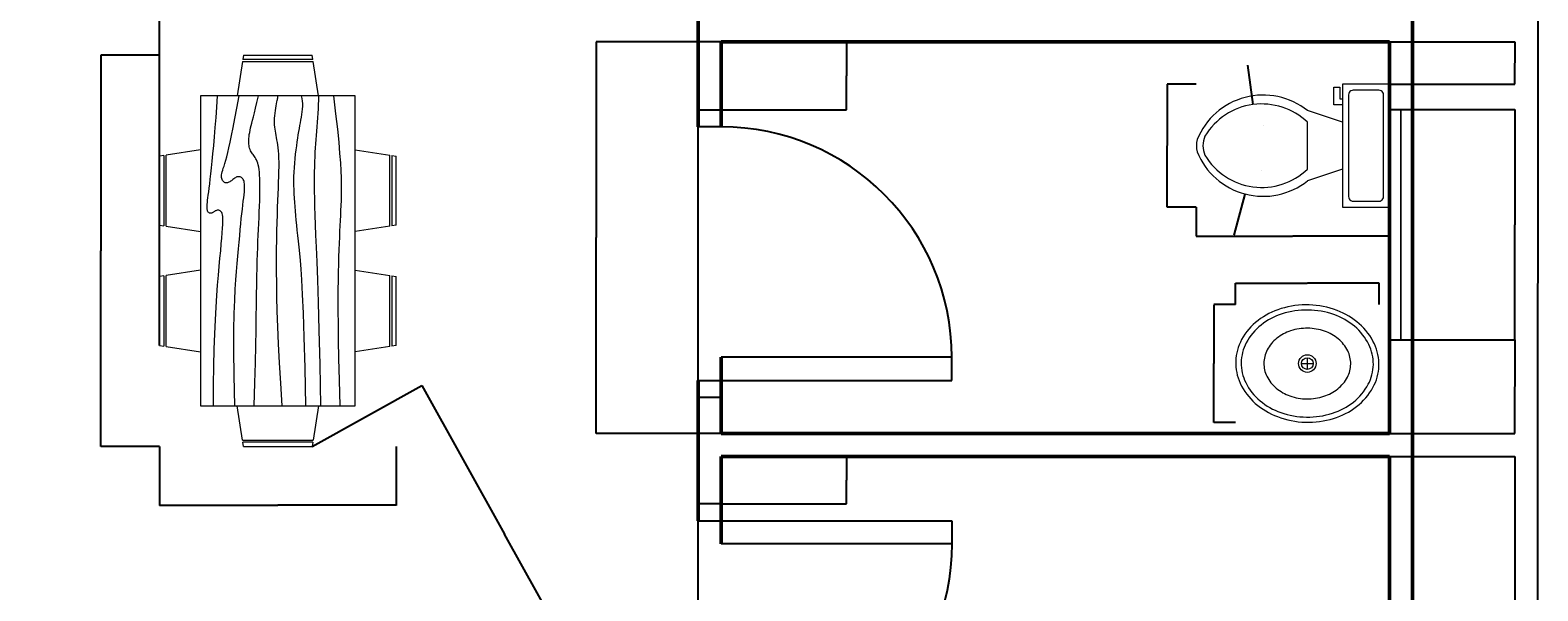
# Model space of a CAD drawing. Units: millimetres. Extents: x 1584 to 12772, y -932 to 10602.
# Tile 3 of 4: x 6228 to 12772, y 3427 to 5860. Entities that reach past the tile are written whole.
import ezdxf

# ---------------------------------------------------------------- set-up
doc = ezdxf.new("R2010")
doc.units = ezdxf.units.MM
for name, color, linetype, lineweight in [('A-ANNO-DIMS', 2, 'Continuous', 18), ('A-DOOR', 3, 'Continuous', 25), ('A-FLOR-FIXT', 9, 'Continuous', 18), ('A-FURN', 8, 'Continuous', 18), ('A-GLAZ', 4, 'Continuous', 18), ('A-WALL', 7, 'Continuous', 50)]:
    doc.layers.add(name, color=color, linetype=linetype, lineweight=lineweight)
doc.styles.get("Standard").update_dxf_attribs({"font": 'arial.ttf'})
doc.dimstyles.get("Standard").update_dxf_attribs({"dimtxt": 0.18, "dimasz": 0.18, "dimexe": 0.18, "dimexo": 0.0625, "dimgap": 0.09, "dimtad": 0, "dimtih": 1, "dimtoh": 1, "dimdec": 4, "dimzin": 0, "dimdsep": 46, "dimtxsty": 'Standard', "dimcen": 0.09, "dimadec": 0, "dimazin": 0, "dimtfac": 1, "dimtdec": 4, "dimtofl": 0, "dimtmove": 0, "dimatfit": 3, "dimfxl": 1, "dimtolj": 1, "dimtzin": 0, "dimarcsym": 0})

# ---------------------------------------------------------------- blocks, each defined once
blk = doc.blocks.new('Dining Set - 36 x 72 in.')
for p, q in [((-22.2343, 26.00059), (-23.4847, 17.99762)), ((-22.2304, 26), (-5.7608, 26)), ((-22, 27.5), (-22.1562, 26.50042)), ((-5.8416, 26.5), (-22.1534, 26.5)), ((-22, 27.5), (-6, 27.5)), ((-5.8437, 26.49966), (-6, 27.5)), ((-4.5152, 17.99762), (-5.7655, 25.99926)), ((5.7657, 26.00059), (4.5153, 17.99762)), ((5.7696, 26), (22.2392, 26)), ((6, 27.5), (5.8438, 26.50042)), ((22.1584, 26.5), (5.8466, 26.5)), ((6, 27.5), (22, 27.5)), ((22.1563, 26.49966), (22, 27.5)), ((23.4848, 17.99762), (22.2345, 25.99926)), ((36, 18), (-36, 18)), ((-36, 18), (-36, -18)), ((36, -18), (36, 18)), ((-45.5, 8), (-44.5004, 8.15617)), ((-45.5, 8), (-45.5, -8)), ((-44.5, -8.15843), (-44.5, 8.15338)), ((-44.0006, 8.23428), (-35.9976, 9.48474)), ((-44, 8.23041), (-44, -8.23915)), ((44.0006, 8.23428), (35.9976, 9.48474)), ((44, 8.23041), (44, -8.23915)), ((44.5, -8.15843), (44.5, 8.15338)), ((45.5, 8), (44.5005, 8.15617)), ((45.5, 8), (45.5, -8)), ((-44.4997, -8.15631), (-45.5, -8)), ((-35.9976, -9.48476), (-43.9993, -8.2345)), ((35.9976, -9.48476), (43.9993, -8.2345)), ((44.4997, -8.15631), (45.5, -8)), ((-36, -18), (36, -18)), ((-22.2343, -26.0006), (-23.4847, -17.99762)), ((-4.5152, -17.99762), (-5.7655, -25.99928)), ((5.7657, -26.0006), (4.5153, -17.99762)), ((23.4848, -17.99762), (22.2345, -25.99928)), ((-22.2304, -26), (-5.7608, -26)), ((-22, -27.5), (-22.1562, -26.50044)), ((-5.8416, -26.5), (-22.1534, -26.5)), ((-22, -27.5), (-6, -27.5)), ((-5.8437, -26.49967), (-6, -27.5)), ((5.7696, -26), (22.2392, -26)), ((6, -27.5), (5.8438, -26.50044)), ((22.1584, -26.5), (5.8466, -26.5)), ((6, -27.5), (22, -27.5)), ((22.1563, -26.49967), (22, -27.5))]:
    blk.add_line(p, q)
for points in [[(-36, 15), (-31.1772, 14.97754), (-26.8079, 14.91406), (-22.8538, 14.81543), (-19.276, 14.6875), (-16.0362, 14.53613), (-13.0957, 14.36718), (-10.4159, 14.18652), (-7.9583, 14), (-5.6904, 13.81315), (-3.6035, 13.63021), (-1.6954, 13.45508), (0.0365, 13.29166), (1.5945, 13.14388), (2.9811, 13.01562), (4.1988, 12.9108), (5.25, 12.83333), (6.1393, 12.78613), (6.8802, 12.76823), (7.4883, 12.77767), (7.9792, 12.8125), (8.3685, 12.87077), (8.6719, 12.95052), (8.9049, 13.0498), (9.0833, 13.16666), (9.2205, 13.29899), (9.3216, 13.44401), (9.3895, 13.59879), (9.4271, 13.76041), (9.4373, 13.92594), (9.4232, 14.09245), (9.3875, 14.257), (9.3333, 14.41666), (9.2638, 14.56917), (9.1836, 14.71484), (9.0975, 14.85465), (9.0104, 14.98958), (8.9272, 15.1206), (8.8529, 15.2487), (8.7922, 15.37483), (8.75, 15.5), (8.7305, 15.62467), (8.7344, 15.74739), (8.7617, 15.86621), (8.8125, 15.97916), (8.8867, 16.08431), (8.9844, 16.17968), (9.1055, 16.26334), (9.25, 16.33333), (9.4189, 16.38802), (9.6172, 16.42708), (9.8506, 16.45052), (10.125, 16.45833), (10.4463, 16.45052), (10.8203, 16.42708), (11.2529, 16.38802), (11.75, 16.33333), (12.3184, 16.26318), (12.9694, 16.17838), (13.7151, 16.07991), (14.5677, 15.96875), (15.5395, 15.84586), (16.6426, 15.71224), (17.8893, 15.56884), (19.2917, 15.41666), (20.859, 15.25667), (22.5879, 15.08984), (24.4721, 14.91715), (26.5052, 14.73958), (28.6809, 14.5581), (30.9929, 14.3737), (33.4347, 14.18733), (36, 14)], [(-36, 10), (-28.9766, 10.14274), (-23.1725, 10.20442), (-18.4241, 10.19775), (-14.5677, 10.13541), (-11.4399, 10.03011), (-8.877, 9.89453), (-6.7154, 9.74137), (-4.7917, 9.58333), (-2.9698, 9.43082), (-1.2246, 9.28515), (0.4415, 9.14534), (2.026, 9.01041), (3.5266, 8.87939), (4.9408, 8.7513), (6.266, 8.62516), (7.5, 8.5), (8.6411, 8.37549), (9.6914, 8.2539), (10.6538, 8.13818), (11.5312, 8.03125), (12.3267, 7.93603), (13.043, 7.85547), (13.6831, 7.79248), (14.25, 7.75), (14.7471, 7.7303), (15.1797, 7.73307), (15.5537, 7.75732), (15.875, 7.80208), (16.1494, 7.86637), (16.3828, 7.94922), (16.5811, 8.04964), (16.75, 8.16666), (16.8944, 8.29915), (17.0143, 8.44531), (17.1089, 8.60319), (17.1771, 8.77083), (17.218, 8.94629), (17.2305, 9.1276), (17.2137, 9.31282), (17.1667, 9.5), (17.0895, 9.6875), (16.987, 9.875), (16.8649, 10.0625), (16.7292, 10.25), (16.5856, 10.4375), (16.4401, 10.625), (16.2985, 10.8125), (16.1667, 11), (16.05, 11.18733), (15.9518, 11.3737), (15.8752, 11.5581), (15.8229, 11.73958), (15.798, 11.91715), (15.8034, 12.08984), (15.842, 12.25667), (15.9167, 12.41666), (16.0295, 12.56836), (16.1784, 12.70833), (16.3605, 12.83268), (16.5729, 12.9375), (16.8127, 13.01888), (17.0768, 13.07291), (17.3625, 13.0957), (17.6667, 13.08333), (17.9894, 13.03312), (18.3418, 12.94726), (18.7382, 12.82918), (19.1927, 12.68229), (19.7195, 12.51001), (20.3327, 12.31575), (21.0465, 12.10294), (21.875, 11.875), (22.8357, 11.63354), (23.959, 11.37304), (25.2786, 11.08618), (26.8282, 10.76562), (28.6414, 10.40405), (30.752, 9.99414), (33.1936, 9.52856), (36, 9)], [(-36, 5.5), (-30.7157, 5.3348), (-26.069, 5.20963), (-21.9946, 5.11767), (-18.4271, 5.05208), (-15.3009, 5.00602), (-12.5508, 4.97265), (-10.1112, 4.94515), (-7.9167, 4.91666), (-5.909, 4.88167), (-4.0586, 4.83984), (-2.3429, 4.79215), (-0.7396, 4.73958), (0.7739, 4.6831), (2.22, 4.6237), (3.6213, 4.56233), (5, 4.5), (6.373, 4.43782), (7.7344, 4.3776), (9.0723, 4.32129), (10.375, 4.27083), (11.6309, 4.22819), (12.8281, 4.19531), (13.9551, 4.17415), (15, 4.16666), (15.954, 4.17448), (16.819, 4.19791), (17.6001, 4.23698), (18.3021, 4.29166), (18.9299, 4.36198), (19.4883, 4.44791), (19.9823, 4.54948), (20.4167, 4.66666), (20.7969, 4.79899), (21.1302, 4.94401), (21.4245, 5.09879), (21.6875, 5.26041), (21.9271, 5.42594), (22.1511, 5.59245), (22.3672, 5.757), (22.5834, 5.91666), (22.8065, 6.06868), (23.0404, 6.21093), (23.2879, 6.34147), (23.5521, 6.45833), (23.8358, 6.55957), (24.142, 6.64323), (24.4735, 6.70735), (24.8334, 6.75), (25.2235, 6.76969), (25.642, 6.76692), (26.0858, 6.74267), (26.5521, 6.69791), (27.0379, 6.63362), (27.5404, 6.55078), (28.0565, 6.45036), (28.5834, 6.33333), (29.1242, 6.19987), (29.7071, 6.04687), (30.3661, 5.87044), (31.1354, 5.66666), (32.0493, 5.43164), (33.142, 5.16146), (34.4475, 4.85221), (36, 4.5)], [(-36, -1), (-30.7915, -0.6591), (-26.0195, -0.38216), (-21.6519, -0.16284), (-17.6563, 0.00521), (-14.0005, 0.12833), (-10.6523, 0.21289), (-7.5796, 0.26522), (-4.75, 0.29166), (-2.134, 0.29793), (0.2878, 0.28711), (2.5317, 0.26163), (4.6146, 0.22396), (6.5529, 0.17651), (8.3633, 0.12174), (10.0623, 0.06209), (11.6667, 0), (13.1899, -0.06201), (14.6341, -0.1211), (15.9982, -0.17432), (17.2813, -0.21875), (18.4823, -0.25147), (19.6003, -0.26953), (20.6343, -0.27002), (21.5834, -0.25), (22.4481, -0.20768), (23.2357, -0.14584), (23.9549, -0.06836), (24.6146, 0.02083), (25.2235, 0.11784), (25.7904, 0.21875), (26.3241, 0.31966), (26.8334, 0.41666), (27.3265, 0.50618), (27.8099, 0.58593), (28.2894, 0.65397), (28.7709, 0.70833), (29.2601, 0.74707), (29.763, 0.76823), (30.2855, 0.76985), (30.8334, 0.75), (31.4088, 0.70784), (31.9994, 0.64713), (32.589, 0.57275), (33.1615, 0.48958), (33.7008, 0.4025), (34.1908, 0.3164), (34.6153, 0.23616), (34.9584, 0.16666), (35.2099, 0.11165), (35.3848, 0.07031), (35.504, 0.04069), (35.5886, 0.02083), (35.6594, 0.00879), (35.7377, 0.0026), (35.8442, 0.00032), (36, 0)], [(-36, -6.5), (-27.1843, -6.31267), (-20.084, -6.1263), (-14.469, -5.9419), (-10.1094, -5.76042), (-6.7752, -5.58285), (-4.2363, -5.41016), (-2.2629, -5.24333), (-0.625, -5.08334), (0.8708, -4.93099), (2.2715, -4.78646), (3.5872, -4.64974), (4.8281, -4.52084), (6.0046, -4.39974), (7.127, -4.28646), (8.2053, -4.18099), (9.25, -4.08334), (10.2705, -3.99382), (11.2734, -3.91407), (12.2647, -3.84603), (13.25, -3.79167), (14.2354, -3.75293), (15.2266, -3.73177), (16.2295, -3.73015), (17.25, -3.75), (18.2912, -3.79248), (19.3451, -3.85547), (20.4009, -3.93604), (21.4479, -4.03125), (22.4754, -4.13819), (23.4727, -4.25391), (24.4289, -4.37549), (25.3334, -4.5), (26.1785, -4.62492), (26.9694, -4.74935), (27.7145, -4.87281), (28.4219, -4.99479), (29.1, -5.11483), (29.7572, -5.23242), (30.4016, -5.34709), (31.0417, -5.45834), (31.6837, -5.56437), (32.3262, -5.65821), (32.9658, -5.73153), (33.599, -5.77604), (34.2224, -5.78345), (34.8327, -5.74545), (35.4264, -5.65373), (36, -5.5)], [(-36, -10), (-26.4022, -9.81299), (-18.4675, -9.62891), (-11.9839, -9.45069), (-6.7396, -9.28125), (-2.5226, -9.12354), (0.8789, -8.98047), (3.6769, -8.85498), (6.0833, -8.75), (8.2767, -8.66765), (10.3021, -8.60677), (12.1712, -8.56543), (13.8958, -8.54167), (15.4876, -8.53353), (16.9583, -8.53907), (18.3197, -8.55632), (19.5834, -8.58334), (20.7616, -8.61841), (21.8685, -8.66081), (22.9188, -8.71004), (23.9271, -8.76563), (24.9081, -8.82707), (25.8763, -8.89388), (26.8465, -8.96558), (27.8334, -9.04167), (28.8474, -9.12118), (29.8828, -9.20117), (30.93, -9.27824), (31.9792, -9.34896), (33.0205, -9.40991), (34.0443, -9.45768), (35.0407, -9.48885), (36, -9.5)], [(-36, -14.5), (-30.0881, -14.33513), (-25.0332, -14.21224), (-20.7312, -14.12647), (-17.0781, -14.07292), (-13.97, -14.04671), (-11.3027, -14.04297), (-8.9724, -14.05681), (-6.875, -14.08334), (-4.9224, -14.11833), (-3.0905, -14.16016), (-1.3709, -14.20785), (0.2448, -14.26042), (1.7647, -14.3169), (3.1973, -14.3763), (4.5507, -14.43767), (5.8333, -14.5), (7.0554, -14.5621), (8.235, -14.62175), (9.3922, -14.67652), (10.5469, -14.72396), (11.7192, -14.76164), (12.929, -14.78711), (14.1965, -14.79794), (15.5417, -14.79167), (16.9933, -14.76424), (18.6152, -14.70508), (20.4804, -14.60197), (22.6615, -14.44271), (25.2312, -14.21509), (28.2624, -13.9069), (31.8277, -13.50594), (36, -13)]]:
    blk.add_lwpolyline(points)
blk = doc.blocks.new('Toilet - top')
for p, q in [((9.5, -6), (9.5, -2)), ((-10, -8.5), (-8, -8.5)), ((-10, -9.5), (-10, -8.5)), ((-7, -9.5), (-10, -9.5)), ((-8, -8.5), (-8, -8)), ((-7, -8), (-7, -9.5)), ((-4, -8), (-6, -14)), ((4, -8), (6, -14)), ((4, -14), (-4, -14))]:
    blk.add_line(p, q)
blk.add_lwpolyline([(10.5, -8), (10.5, 0), (-10.5, 0), (-10.5, -8)], close=True)
for points in [[(-9.5, -2), (-9.5, -6)], [(8.5, -1), (-8.5, -1)], [(-8.5, -7), (8.5, -7)]]:
    blk.add_lwpolyline(points)
for centre, radius, start, end in [((-8.62, -1.88), 0.884, 81.8699, 188.1301), ((8.62, -1.88), 0.884, 351.8699, 98.1301), ((-8.62, -6.12), 0.884, 171.8699, 278.1301), ((8.62, -6.12), 0.884, 261.8699, 8.1301), ((3.52, -21.58), 12.17, 141.4691, 247.9714), ((4.2, -21.82), 11.33, 136.3677, 238.9468), ((-3.52, -21.58), 12.17, 292.0284, 38.5307), ((-4.2, -21.82), 11.33, 301.053, 43.6321), ((0, -27.88), 4, 245.7318, 294.2682), ((0, -29), 4, 254.8605, 285.1395)]:
    blk.add_arc(centre, radius, start, end)
blk = doc.blocks.new('Sink - Oval top')
for p, q in [((-1, 0), (1, 0)), ((0, 1), (0, -1))]:
    blk.add_line(p, q)
for points in [[(-12.23, 0.39, 0.117634), (-11.46, -3.36, 0.104469), (-8.88, -6.8, 0.090016), (-5.08, -9.07, 0.08192), (-0.32, -10.02, 0.08192), (4.49, -9.38, 0.090016), (8.42, -7.36, 0.104469), (11.22, -4.09, 0.117634), (12.23, -0.39, 0.117634), (11.46, 3.36, 0.104469), (8.88, 6.8, 0.090016), (5.08, 9.07, 0.08192), (0.32, 10.02, 0.08192), (-4.49, 9.38, 0.090016), (-8.42, 7.36, 0.104469), (-11.22, 4.09, 0.117634)], [(-11.29, 0.16, 0.118622), (-10.52, -3.25, 0.104678), (-8.07, -6.36, 0.089562), (-4.54, -8.37, 0.081185), (-0.13, -9.15, 0.081185), (4.3, -8.49, 0.089562), (7.89, -6.58, 0.104678), (10.42, -3.55, 0.118622), (11.29, -0.16, 0.118622), (10.52, 3.25, 0.104678), (8.07, 6.36, 0.089562), (4.54, 8.37, 0.081185), (0.13, 9.15, 0.081185), (-4.3, 8.49, 0.089562), (-7.89, 6.58, 0.104678), (-10.42, 3.55, 0.118622)], [(-7.42, 0.08, 0.118283), (-6.91, -2.17, 0.104607), (-5.29, -4.21, 0.089718), (-2.97, -5.53, 0.081436), (-0.07, -6.04, 0.081436), (2.84, -5.59, 0.089718), (5.2, -4.33, 0.104607), (6.86, -2.32, 0.118283), (7.42, -0.08, 0.118283), (6.91, 2.17, 0.104607), (5.29, 4.21, 0.089718), (2.97, 5.53, 0.081436), (0.07, 6.04, 0.081436), (-2.84, 5.59, 0.089718), (-5.2, 4.33, 0.104607), (-6.86, 2.32, 0.118283)]]:
    blk.add_lwpolyline(points, format="xyb", close=True)
for radius in [1.5, 1]:
    blk.add_circle((0, 0), radius)
blk = doc.blocks.new('DOOR-SINGLE-1000')
for p, q in [((1000, 1174.2), (1000, 1248.4)), ((1000, 1248.4), (1100, 1248.4)), ((1100, 1248.4), (1100, 1174.2)), ((1000, 1174.2), (0, 1174.2)), ((0, 1174.2), (0, 1074.2)), ((1000, 1074.2), (1000, 1174.2)), ((1100, 1174.2), (1000, 1174.2)), ((0, 1074.2), (1000, 1074.2)), ((1000, 0), (1000, 74.2)), ((1000, 74.2), (1100, 74.2)), ((1100, 74.2), (1100, 0)), ((1100, 0), (1000, 0))]:
    blk.add_line(p, q)
blk.add_arc((1000, 1074.2), 1000, 180, 270)
blk = doc.blocks.new('*D28')
at = {"layer": 'A-ANNO-DIMS', "color": 0, "lineweight": -2, "transparency": 16777216}
for p, q in [((6789.5, 5751.9), (6534.6, 5751.9)), ((6534.8, 5751.7), (6534.8, 4902.6)), ((6534.8, 4053.1), (6534.8, 4902.2)), ((6789.5, 4053), (6534.6, 4053))]:
    blk.add_line(p, q, dxfattribs=at)
at = {"layer": 'A-ANNO-DIMS', "color": 0, "transparency": 16777216}
for points in [[(6534.7, 5751.7), (6534.8, 5751.7), (6534.8, 5751.9)], [(6534.7, 4053.1), (6534.8, 4053.1), (6534.8, 4053)]]:
    blk.add_solid(points, dxfattribs=at)
at = {"layer": 'Defpoints', "color": 0, "transparency": 16777216}
for p in [(6534.8, 5751.9), (6789.6, 5751.9), (6789.6, 4053)]:
    blk.add_point(p, dxfattribs=at)
at = {"layer": 'A-ANNO-DIMS', "color": 0, "transparency": 16777216, "insert": (6534.8, 4902.4), "char_height": 0.18, "attachment_point": 5}
blk.add_mtext('\\A1;DINING SET 1699', dxfattribs=at)
blk = doc.blocks.new('*D29')
at = {"layer": 'A-ANNO-DIMS', "color": 0, "lineweight": -2, "transparency": 16777216}
for p, q in [((6789.6, 4052.9), (6789.6, 3797.9)), ((7816.4, 4052.9), (7816.4, 3797.9)), ((6789.8, 3798.1), (7302.6, 3798.1)), ((7816.2, 3798.1), (7303.3, 3798.1))]:
    blk.add_line(p, q, dxfattribs=at)
at = {"layer": 'A-ANNO-DIMS', "color": 0, "transparency": 16777216}
for points in [[(6789.8, 3798.2), (6789.8, 3798.1), (6789.6, 3798.1)], [(7816.2, 3798.2), (7816.2, 3798.1), (7816.4, 3798.1)]]:
    blk.add_solid(points, dxfattribs=at)
at = {"layer": 'Defpoints', "color": 0, "transparency": 16777216}
for p in [(6789.6, 4053), (7816.4, 4053), (6789.6, 3798.1)]:
    blk.add_point(p, dxfattribs=at)
at = {"layer": 'A-ANNO-DIMS', "color": 0, "transparency": 16777216, "insert": (7303, 3798.1), "char_height": 0.18, "attachment_point": 5}
blk.add_mtext('\\A1;1027', dxfattribs=at)
blk = doc.blocks.new('*D32')
at = {"layer": 'A-ANNO-DIMS', "color": 0, "lineweight": -2, "transparency": 16777216}
for p, q in [((11288.5, 5091.9), (11288.5, 4965.9)), ((12127.8, 5091.9), (12127.8, 4965.9)), ((11288.6, 4966.1), (11707.6, 4966.1)), ((12127.7, 4966.1), (11708.7, 4966.1))]:
    blk.add_line(p, q, dxfattribs=at)
at = {"layer": 'A-ANNO-DIMS', "color": 0, "transparency": 16777216}
for points in [[(11288.6, 4966.1), (11288.6, 4966.1), (11288.5, 4966.1)], [(12127.7, 4966.1), (12127.7, 4966.1), (12127.8, 4966.1)]]:
    blk.add_solid(points, dxfattribs=at)
at = {"layer": 'Defpoints', "color": 0, "transparency": 16777216}
for p in [(11288.5, 5092), (12127.8, 5092), (12127.8, 4966.1)]:
    blk.add_point(p, dxfattribs=at)
at = {"layer": 'A-ANNO-DIMS', "color": 0, "transparency": 16777216, "insert": (11708.1, 4966.1), "char_height": 0.18, "attachment_point": 5}
blk.add_mtext('\\A1;WC 839', dxfattribs=at)
blk = doc.blocks.new('*D33')
at = {"layer": 'A-ANNO-DIMS', "color": 0, "lineweight": -2, "transparency": 16777216}
for p, q in [((11288.4, 5625.4), (11162.4, 5625.4)), ((11162.6, 5625.2), (11162.6, 5358.9)), ((11162.6, 5092.2), (11162.6, 5358.5)), ((11288.4, 5092), (11162.4, 5092))]:
    blk.add_line(p, q, dxfattribs=at)
at = {"layer": 'A-ANNO-DIMS', "color": 0, "transparency": 16777216}
for points in [[(11162.5, 5625.2), (11162.6, 5625.2), (11162.6, 5625.4)], [(11162.5, 5092.2), (11162.6, 5092.2), (11162.6, 5092)]]:
    blk.add_solid(points, dxfattribs=at)
at = {"layer": 'Defpoints', "color": 0, "transparency": 16777216}
for p in [(11288.5, 5625.4), (11162.6, 5092), (11288.5, 5092)]:
    blk.add_point(p, dxfattribs=at)
at = {"layer": 'A-ANNO-DIMS', "color": 0, "transparency": 16777216, "insert": (11162.6, 5358.7), "char_height": 0.18, "attachment_point": 5}
blk.add_mtext('\\A1;533', dxfattribs=at)
blk = doc.blocks.new('*D34')
at = {"layer": 'A-ANNO-DIMS', "color": 0, "lineweight": -2, "transparency": 16777216}
for p, q in [((11459.3, 4669.1), (11459.3, 4762.7)), ((11459.5, 4762.5), (11770.4, 4762.5)), ((12082.7, 4762.5), (11771.8, 4762.5)), ((12082.9, 4669.1), (12082.9, 4762.7))]:
    blk.add_line(p, q, dxfattribs=at)
at = {"layer": 'A-ANNO-DIMS', "color": 0, "transparency": 16777216}
for points in [[(11459.5, 4762.6), (11459.5, 4762.5), (11459.3, 4762.5)], [(12082.7, 4762.6), (12082.7, 4762.5), (12082.9, 4762.5)]]:
    blk.add_solid(points, dxfattribs=at)
at = {"layer": 'Defpoints', "color": 0, "transparency": 16777216}
for p in [(12082.9, 4762.5), (11459.3, 4669), (12082.9, 4669)]:
    blk.add_point(p, dxfattribs=at)
at = {"layer": 'A-ANNO-DIMS', "color": 0, "transparency": 16777216, "insert": (11771.1, 4762.5), "char_height": 0.18, "attachment_point": 5}
blk.add_mtext('\\A1;BASIN 624', dxfattribs=at)
blk = doc.blocks.new('*D35')
at = {"layer": 'A-ANNO-DIMS', "color": 0, "lineweight": -2, "transparency": 16777216}
for p, q in [((11459.3, 4669), (11365.6, 4669)), ((11365.8, 4668.8), (11365.8, 4413.4)), ((11365.8, 4157.7), (11365.8, 4413.1)), ((11459.3, 4157.5), (11365.6, 4157.5))]:
    blk.add_line(p, q, dxfattribs=at)
at = {"layer": 'A-ANNO-DIMS', "color": 0, "transparency": 16777216}
for points in [[(11365.8, 4668.8), (11365.8, 4668.8), (11365.8, 4669)], [(11365.8, 4157.7), (11365.8, 4157.7), (11365.8, 4157.5)]]:
    blk.add_solid(points, dxfattribs=at)
at = {"layer": 'Defpoints', "color": 0, "transparency": 16777216}
for p in [(11365.8, 4669), (11459.3, 4669), (11459.3, 4157.5)]:
    blk.add_point(p, dxfattribs=at)
at = {"layer": 'A-ANNO-DIMS', "color": 0, "transparency": 16777216, "insert": (11365.8, 4413.3), "char_height": 0.18, "attachment_point": 5}
blk.add_mtext('\\A1;511', dxfattribs=at)
blk = doc.blocks.new('*D37')
at = {"layer": 'A-ANNO-DIMS', "color": 0, "lineweight": -2, "transparency": 16777216}
for p, q in [((12227.9, 9910.2), (12771.7, 9910.2)), ((12771.5, 9910), (12771.5, 4761.5)), ((12771.5, -387.5), (12771.5, 4761.1)), ((8227.9, -387.6), (12771.7, -387.6))]:
    blk.add_line(p, q, dxfattribs=at)
at = {"layer": 'A-ANNO-DIMS', "color": 0, "transparency": 16777216}
for points in [[(12771.5, 9910), (12771.6, 9910), (12771.5, 9910.2)], [(12771.5, -387.5), (12771.6, -387.5), (12771.5, -387.6)]]:
    blk.add_solid(points, dxfattribs=at)
at = {"layer": 'Defpoints', "color": 0, "transparency": 16777216}
for p in [(12227.8, 9910.2), (12771.5, 9910.2), (8227.8, -387.6)]:
    blk.add_point(p, dxfattribs=at)
at = {"layer": 'A-ANNO-DIMS', "color": 0, "transparency": 16777216, "insert": (12771.5, 4761.3), "char_height": 0.18, "attachment_point": 5}
blk.add_mtext('\\A1;10298', dxfattribs=at)
blk = doc.blocks.new('*D41')
at = {"layer": 'A-ANNO-DIMS', "color": 0, "lineweight": -2, "transparency": 16777216}
for p, q in [((12127.9, 4010.2), (12671.7, 4010.2)), ((12671.5, 4010), (12671.5, 3306.6)), ((12671.5, 2602.8), (12671.5, 3306.2)), ((12127.9, 2602.6), (12671.7, 2602.6))]:
    blk.add_line(p, q, dxfattribs=at)
at = {"layer": 'A-ANNO-DIMS', "color": 0, "transparency": 16777216}
for points in [[(12671.5, 4010), (12671.6, 4010), (12671.5, 4010.2)], [(12671.5, 2602.8), (12671.6, 2602.8), (12671.5, 2602.6)]]:
    blk.add_solid(points, dxfattribs=at)
at = {"layer": 'Defpoints', "color": 0, "transparency": 16777216}
for p in [(12127.8, 4010.2), (12127.8, 2602.6), (12671.5, 2602.6)]:
    blk.add_point(p, dxfattribs=at)
at = {"layer": 'A-ANNO-DIMS', "color": 0, "transparency": 16777216, "insert": (12671.5, 3306.4), "char_height": 0.18, "attachment_point": 5}
blk.add_mtext('\\A1;1407.6', dxfattribs=at)
blk = doc.blocks.new('*D42')
at = {"layer": 'A-ANNO-DIMS', "color": 0, "lineweight": -2, "transparency": 16777216}
for p, q in [((9227.8, 5810.2), (8684, 5810.2)), ((8684.1, 5810), (8684.1, 4960.4)), ((8684.1, 4110.4), (8684.1, 4960)), ((9227.8, 4110.2), (8684, 4110.2))]:
    blk.add_line(p, q, dxfattribs=at)
at = {"layer": 'A-ANNO-DIMS', "color": 0, "transparency": 16777216}
for points in [[(8684.1, 5810), (8684.2, 5810), (8684.1, 5810.2)], [(8684.1, 4110.4), (8684.2, 4110.4), (8684.1, 4110.2)]]:
    blk.add_solid(points, dxfattribs=at)
at = {"layer": 'Defpoints', "color": 0, "transparency": 16777216}
for p in [(8684.1, 5810.2), (9227.8, 5810.2), (9227.8, 4110.2)]:
    blk.add_point(p, dxfattribs=at)
at = {"layer": 'A-ANNO-DIMS', "color": 0, "transparency": 16777216, "insert": (8684.1, 4960.2), "char_height": 0.18, "attachment_point": 5}
blk.add_mtext('\\A1;1700', dxfattribs=at)
blk = doc.blocks.new('*D44')
at = {"layer": 'A-ANNO-DIMS', "color": 0, "lineweight": -2, "transparency": 16777216}
for p, q in [((5227.8, 312.4), (5227.8, 10454.1)), ((5228, 10453.9), (7177.5, 10453.9)), ((9127.7, 10453.9), (7178.2, 10453.9)), ((9127.8, 312.4), (9127.8, 10454.1))]:
    blk.add_line(p, q, dxfattribs=at)
at = {"layer": 'A-ANNO-DIMS', "color": 0, "transparency": 16777216}
for points in [[(5228, 10453.9), (5228, 10453.9), (5227.8, 10453.9)], [(9127.7, 10453.9), (9127.7, 10453.9), (9127.8, 10453.9)]]:
    blk.add_solid(points, dxfattribs=at)
at = {"layer": 'Defpoints', "color": 0, "transparency": 16777216}
for p in [(9127.8, 10453.9), (5227.8, 312.4), (9127.8, 312.4)]:
    blk.add_point(p, dxfattribs=at)
at = {"layer": 'A-ANNO-DIMS', "color": 0, "transparency": 16777216, "insert": (7177.8, 10453.9), "char_height": 0.18, "attachment_point": 5}
blk.add_mtext('\\A1;3900', dxfattribs=at)
blk = doc.blocks.new('*D59')
at = {"layer": 'A-ANNO-DIMS', "color": 0, "lineweight": -2, "transparency": 16777216}
for p, q in [((9227.9, 5810.2), (9771.7, 5810.2)), ((9771.5, 5810), (9771.5, 5662.5)), ((9771.5, 5514.7), (9771.5, 5662.2)), ((9227.9, 5514.5), (9771.7, 5514.5))]:
    blk.add_line(p, q, dxfattribs=at)
at = {"layer": 'A-ANNO-DIMS', "color": 0, "transparency": 16777216}
for points in [[(9771.5, 5810), (9771.6, 5810), (9771.5, 5810.2)], [(9771.5, 5514.7), (9771.6, 5514.7), (9771.5, 5514.5)]]:
    blk.add_solid(points, dxfattribs=at)
at = {"layer": 'Defpoints', "color": 0, "transparency": 16777216}
for p in [(9227.8, 5810.2), (9227.8, 5514.5), (9771.5, 5514.5)]:
    blk.add_point(p, dxfattribs=at)
at = {"layer": 'A-ANNO-DIMS', "color": 0, "transparency": 16777216, "insert": (9771.5, 5662.3), "char_height": 0.18, "attachment_point": 5}
blk.add_mtext('\\A1;295.7', dxfattribs=at)
blk = doc.blocks.new('*D60')
at = {"layer": 'A-ANNO-DIMS', "color": 0, "lineweight": -2, "transparency": 16777216}
for p, q in [((9227.9, 4010.2), (9771.7, 4010.2)), ((9771.5, 4010), (9771.5, 3907.5)), ((9771.5, 3804.6), (9771.5, 3907.1)), ((9227.9, 3804.4), (9771.7, 3804.4))]:
    blk.add_line(p, q, dxfattribs=at)
at = {"layer": 'A-ANNO-DIMS', "color": 0, "transparency": 16777216}
for points in [[(9771.5, 4010), (9771.6, 4010), (9771.5, 4010.2)], [(9771.5, 3804.6), (9771.6, 3804.6), (9771.5, 3804.4)]]:
    blk.add_solid(points, dxfattribs=at)
at = {"layer": 'Defpoints', "color": 0, "transparency": 16777216}
for p in [(9227.8, 4010.2), (9227.8, 3804.4), (9771.5, 3804.4)]:
    blk.add_point(p, dxfattribs=at)
at = {"layer": 'A-ANNO-DIMS', "color": 0, "transparency": 16777216, "insert": (9771.5, 3907.3), "char_height": 0.18, "attachment_point": 5}
blk.add_mtext('\\A1;205.8', dxfattribs=at)
blk = doc.blocks.new('*D69')
at = {"layer": 'A-ANNO-DIMS', "color": 0, "lineweight": -2, "transparency": 16777216}
for p, q in [((12127.9, 5515.7), (12671.7, 5515.7)), ((12671.5, 5515.5), (12671.5, 5015.9)), ((12671.5, 4515.9), (12671.5, 5015.5)), ((12127.9, 4515.7), (12671.7, 4515.7))]:
    blk.add_line(p, q, dxfattribs=at)
at = {"layer": 'A-ANNO-DIMS', "color": 0, "transparency": 16777216}
for points in [[(12671.5, 5515.5), (12671.6, 5515.5), (12671.5, 5515.7)], [(12671.5, 4515.9), (12671.6, 4515.9), (12671.5, 4515.7)]]:
    blk.add_solid(points, dxfattribs=at)
at = {"layer": 'Defpoints', "color": 0, "transparency": 16777216}
for p in [(12127.8, 5515.7), (12127.8, 4515.7), (12671.5, 4515.7)]:
    blk.add_point(p, dxfattribs=at)
at = {"layer": 'A-ANNO-DIMS', "color": 0, "transparency": 16777216, "insert": (12671.5, 5015.7), "char_height": 0.18, "attachment_point": 5}
blk.add_mtext('\\A1;1000', dxfattribs=at)
blk = doc.blocks.new('*D70')
at = {"layer": 'A-ANNO-DIMS', "color": 0, "lineweight": -2, "transparency": 16777216}
for p, q in [((12127.9, 4515.7), (12671.7, 4515.7)), ((12671.5, 4515.5), (12671.5, 4313.1)), ((12671.5, 4110.4), (12671.5, 4312.8)), ((12127.9, 4110.2), (12671.7, 4110.2))]:
    blk.add_line(p, q, dxfattribs=at)
at = {"layer": 'A-ANNO-DIMS', "color": 0, "transparency": 16777216}
for points in [[(12671.5, 4515.5), (12671.6, 4515.5), (12671.5, 4515.7)], [(12671.5, 4110.4), (12671.6, 4110.4), (12671.5, 4110.2)]]:
    blk.add_solid(points, dxfattribs=at)
at = {"layer": 'Defpoints', "color": 0, "transparency": 16777216}
for p in [(12127.8, 4515.7), (12127.8, 4110.2), (12671.5, 4110.2)]:
    blk.add_point(p, dxfattribs=at)
at = {"layer": 'A-ANNO-DIMS', "color": 0, "transparency": 16777216, "insert": (12671.5, 4312.9), "char_height": 0.18, "attachment_point": 5}
blk.add_mtext('\\A1;405.5', dxfattribs=at)
blk = doc.blocks.new('*D71')
at = {"layer": 'A-ANNO-DIMS', "color": 0, "lineweight": -2, "transparency": 16777216}
for p, q in [((12127.9, 5810.2), (12671.7, 5810.2)), ((12671.5, 5810), (12671.5, 5718)), ((12671.5, 5625.6), (12671.5, 5717.6)), ((12127.9, 5625.4), (12671.7, 5625.4))]:
    blk.add_line(p, q, dxfattribs=at)
at = {"layer": 'A-ANNO-DIMS', "color": 0, "transparency": 16777216}
for points in [[(12671.5, 5810), (12671.6, 5810), (12671.5, 5810.2)], [(12671.5, 5625.6), (12671.6, 5625.6), (12671.5, 5625.4)]]:
    blk.add_solid(points, dxfattribs=at)
at = {"layer": 'Defpoints', "color": 0, "transparency": 16777216}
for p in [(12127.8, 5810.2), (12127.8, 5625.4), (12671.5, 5625.4)]:
    blk.add_point(p, dxfattribs=at)
at = {"layer": 'A-ANNO-DIMS', "color": 0, "transparency": 16777216, "insert": (12671.5, 5717.8), "char_height": 0.18, "attachment_point": 5}
blk.add_mtext('\\A1;184.77', dxfattribs=at)
blk = doc.blocks.new('*D72')
at = {"layer": 'A-ANNO-DIMS', "color": 0, "lineweight": -2, "transparency": 16777216}
for p, q in [((5227.8, 4479), (5227.8, 10454.1)), ((5228, 10453.9), (6008.3, 10453.9)), ((6789.4, 10453.9), (6009.2, 10453.9)), ((6789.6, 4491.7), (6789.6, 10454.1))]:
    blk.add_line(p, q, dxfattribs=at)
at = {"layer": 'A-ANNO-DIMS', "color": 0, "transparency": 16777216}
for points in [[(5228, 10453.9), (5228, 10453.9), (5227.8, 10453.9)], [(6789.4, 10453.9), (6789.4, 10453.9), (6789.6, 10453.9)]]:
    blk.add_solid(points, dxfattribs=at)
at = {"layer": 'Defpoints', "color": 0, "transparency": 16777216}
for p in [(6789.6, 10453.9), (5227.8, 4478.9), (6789.6, 4491.7)]:
    blk.add_point(p, dxfattribs=at)
at = {"layer": 'A-ANNO-DIMS', "color": 0, "transparency": 16777216, "insert": (6008.7, 10453.9), "char_height": 0.18, "attachment_point": 5}
blk.add_mtext('\\A1;1561.8', dxfattribs=at)
blk = doc.blocks.new('*D73')
at = {"layer": 'A-ANNO-DIMS', "color": 0, "lineweight": -2, "transparency": 16777216}
for p, q in [((7452.4, 4053), (7927.2, 4318.1)), ((7927.2, 4317.8), (8287.2, 3672.9)), ((8647.5, 3027.5), (8287.4, 3672.5)), ((8172.9, 2762.4), (8647.7, 3027.5))]:
    blk.add_line(p, q, dxfattribs=at)
at = {"layer": 'A-ANNO-DIMS', "color": 0, "transparency": 16777216}
for points in [[(7927.2, 4317.8), (7927.1, 4317.8), (7927.1, 4318)], [(8647.5, 3027.6), (8647.4, 3027.5), (8647.6, 3027.4)]]:
    blk.add_solid(points, dxfattribs=at)
at = {"layer": 'Defpoints', "color": 0, "transparency": 16777216}
for p in [(7452.3, 4053), (8647.6, 3027.4), (8172.8, 2762.4)]:
    blk.add_point(p, dxfattribs=at)
at = {"layer": 'A-ANNO-DIMS', "color": 0, "transparency": 16777216, "insert": (8287.3, 3672.7), "char_height": 0.18, "attachment_point": 5}
blk.add_mtext('\\A1;1478', dxfattribs=at)
blk = doc.blocks.new('*D85')
at = {"layer": 'A-ANNO-DIMS', "color": 0, "lineweight": -2, "transparency": 16777216}
for p, q in [((11579.6, 5448.1), (11579.8, 5448.1)), ((11579.7, 5448), (11579.7, 5448.2)), ((11454, 4969.8), (11501.1, 5149)), ((11453.8, 4969.8), (11454, 4969.8))]:
    blk.add_line(p, q, dxfattribs=at)
at = {"layer": 'A-ANNO-DIMS', "color": 0, "transparency": 16777216}
blk.add_solid([(11501.1, 5149), (11501.1, 5149), (11501.1, 5149.2)], dxfattribs=at)
at = {"layer": 'Defpoints', "color": 0, "transparency": 16777216}
for p in [(11579.7, 5448.1), (11501.1, 5149.2)]:
    blk.add_point(p, dxfattribs=at)
at = {"layer": 'A-ANNO-DIMS', "color": 0, "transparency": 16777216, "insert": (11453.2, 4969.8), "char_height": 0.18, "attachment_point": 5}
blk.add_mtext('\\A1;2X R309.1', dxfattribs=at)
blk = doc.blocks.new('*D86')
at = {"layer": 'A-ANNO-DIMS', "color": 0, "lineweight": -2, "transparency": 16777216}
for p, q in [((11512.1, 5708.3), (11512.3, 5708.3)), ((11512.3, 5708.3), (11535.3, 5537.4)), ((11573.6, 5252), (11573.8, 5252)), ((11573.7, 5251.9), (11573.7, 5252.1))]:
    blk.add_line(p, q, dxfattribs=at)
at = {"layer": 'A-ANNO-DIMS', "color": 0, "transparency": 16777216}
blk.add_solid([(11535.3, 5537.4), (11535.3, 5537.4), (11535.3, 5537.2)], dxfattribs=at)
at = {"layer": 'Defpoints', "color": 0, "transparency": 16777216}
for p in [(11535.3, 5537.2), (11573.7, 5252)]:
    blk.add_point(p, dxfattribs=at)
at = {"layer": 'A-ANNO-DIMS', "color": 0, "transparency": 16777216, "insert": (11511.4, 5708.3), "char_height": 0.18, "attachment_point": 5}
blk.add_mtext('\\A1;2X R287.76', dxfattribs=at)

msp = doc.modelspace()

# ---------------------------------------------------------------- linework, layer by layer
at = {"layer": 'A-GLAZ'}
for p, q in [((12127.833, 4515.694), (12127.833, 5515.694)), ((12127.833, 5515.694), (12227.833, 5515.694)), ((12177.833, 5515.694), (12177.833, 4515.694)), ((12177.833, 4515.694), (12177.833, 5515.694)), ((12227.833, 5515.694), (12227.833, 4515.694)), ((12227.833, 5515.694), (12227.833, 4515.694)), ((12227.833, 4515.694), (12127.833, 4515.694))]:
    msp.add_line(p, q, dxfattribs=at)
at = {"layer": 'A-WALL'}
for p, q in [((12227.833, 9910.181), (12227.833, 810.181)), ((9127.833, 5910.181), (9127.833, 5810.181)), ((9127.833, 5810.181), (9127.833, 5440.297)), ((9227.833, 5810.181), (12127.833, 5810.181)), ((9227.833, 5810.181), (9227.833, 5440.297)), ((12127.833, 5810.181), (12127.833, 4110.181)), ((9227.833, 4440.297), (9227.833, 4110.181)), ((9127.833, 4340.297), (9127.833, 3730.192)), ((12127.833, 4110.181), (9227.833, 4110.181)), ((12127.833, 4010.181), (9227.833, 4010.181)), ((9227.833, 4010.181), (9227.833, 3630.192)), ((12127.833, 4010.181), (12127.833, 910.181))]:
    msp.add_line(p, q, dxfattribs=at)

# ---------------------------------------------------------------- block references
at = {"layer": 'A-DOOR', "rotation": 180}
msp.add_blockref('DOOR-SINGLE-1000', (10227.833, 5514.497), dxfattribs=at)
at = {"layer": 'A-DOOR', "extrusion": (0, 0, -1), "zscale": -1}
msp.add_blockref('DOOR-SINGLE-1000', (-10227.833, 2555.992), dxfattribs=at)
at = {"layer": 'A-FLOR-FIXT', "xscale": 25.4, "yscale": 25.4, "zscale": 25.4, "rotation": 270}
msp.add_blockref('Toilet - top', (12127.833, 5358.711), dxfattribs=at)
at = {"layer": 'A-FLOR-FIXT', "xscale": 25.4, "yscale": 25.4, "zscale": 25.4}
msp.add_blockref('Sink - Oval top', (11771.13, 4413.261), dxfattribs=at)
at = {"layer": 'A-FURN', "xscale": 18.66924539286349, "yscale": 18.66924539286349, "zscale": 18.66924539286349, "rotation": 90}
msp.add_blockref('Dining Set - 36 x 72 in.', (7302.993, 4902.408), dxfattribs=at)

# ---------------------------------------------------------------- dimensions: what is measured, and where the dimension line sits
at = {"layer": 'A-ANNO-DIMS'}
for base, p1, p2, override, picture, middle in [((9127.833, 10453.881), (5227.833, 312.362), (9127.833, 312.362), {"dimdec": 0, "dimlfac": 1, "dimrnd": 0, "dimzin": 0, "dimdsep": 46, "dimlunit": 2}, '*D44', (7177.833, 10453.881)), ((6789.588, 10453.881), (5227.833, 4478.914), (6789.588, 4491.685), {"dimdec": 1, "dimlfac": 1, "dimrnd": 0, "dimzin": 0, "dimdsep": 46, "dimlunit": 2}, '*D72', (6008.711, 10453.881))]:
    dim = msp.add_linear_dim(base=base, p1=p1, p2=p2, dimstyle='Standard', override=override, dxfattribs=at)
    dim.commit()
    dim.dimension.update_dxf_attribs({"geometry": picture, "text_midpoint": middle})
for base, p1, p2, angle, override, picture, middle in [((12771.533, 9910.181), (8227.833, -387.638), (12227.833, 9910.181), 90, {"dimdec": 0, "dimlfac": 1, "dimrnd": 0, "dimzin": 0, "dimdsep": 46, "dimlunit": 2}, '*D37', (12771.533, 4761.271)), ((8684.133, 5810.181), (9227.833, 4110.181), (9227.833, 5810.181), 90, {"dimdec": 0, "dimlfac": 1, "dimrnd": 0, "dimzin": 0, "dimdsep": 46, "dimlunit": 2}, '*D42', (8684.133, 4960.181)), ((9771.533, 5514.497), (9227.833, 5810.181), (9227.833, 5514.497), 270, {"dimdec": 1, "dimlfac": 1, "dimrnd": 0, "dimzin": 0, "dimdsep": 46, "dimlunit": 2}, '*D59', (9771.533, 5662.339)), ((12671.533, 5625.411), (12127.833, 5810.181), (12127.833, 5625.411), 270, {"dimdec": 2, "dimlfac": 1, "dimrnd": 0, "dimzin": 0, "dimdsep": 46, "dimlunit": 2}, '*D71', (12671.533, 5717.796)), ((11162.552, 5092.011), (11288.459, 5625.411), (11288.459, 5092.011), 270, {"dimdec": 0, "dimlfac": 1, "dimrnd": 0, "dimzin": 0, "dimdsep": 46, "dimlunit": 2}, '*D33', (11162.552, 5358.711)), ((12671.533, 4515.694), (12127.833, 5515.694), (12127.833, 4515.694), 270, {"dimdec": 0, "dimlfac": 1, "dimrnd": 0, "dimzin": 0, "dimdsep": 46, "dimlunit": 2}, '*D69', (12671.533, 5015.694)), ((11365.795, 4668.996), (11459.334, 4157.526), (11459.334, 4668.996), 90, {"dimdec": 0, "dimlfac": 1, "dimrnd": 0, "dimzin": 0, "dimdsep": 46, "dimlunit": 2}, '*D35', (11365.795, 4413.261)), ((12671.533, 4110.181), (12127.833, 4515.694), (12127.833, 4110.181), 270, {"dimdec": 1, "dimlfac": 1, "dimrnd": 0, "dimzin": 0, "dimdsep": 46, "dimlunit": 2}, '*D70', (12671.533, 4312.937)), ((8647.556, 3027.383), (7452.347, 4052.958), (8172.821, 2762.362), 299.1724058, {"dimdec": 0, "dimlfac": 1, "dimrnd": 0, "dimzin": 0, "dimdsep": 46, "dimlunit": 2}, '*D73', (8287.319, 3672.68)), ((6789.588, 3798.122), (7816.397, 4052.958), (6789.588, 4052.958), 180, {"dimdec": 0, "dimlfac": 1, "dimrnd": 0, "dimzin": 0, "dimdsep": 46, "dimlunit": 2}, '*D29', (7302.993, 3798.122)), ((9771.533, 3804.392), (9227.833, 4010.181), (9227.833, 3804.392), 270, {"dimdec": 1, "dimlfac": 1, "dimrnd": 0, "dimzin": 0, "dimdsep": 46, "dimlunit": 2}, '*D60', (9771.533, 3907.286)), ((12671.533, 2602.614), (12127.833, 4010.181), (12127.833, 2602.614), 270, {"dimdec": 1, "dimlfac": 1, "dimrnd": 0, "dimzin": 0, "dimdsep": 46, "dimlunit": 2}, '*D41', (12671.533, 3306.397))]:
    dim = msp.add_linear_dim(base=base, p1=p1, p2=p2, angle=angle, dimstyle='Standard', override=override, dxfattribs=at)
    dim.commit()
    dim.dimension.update_dxf_attribs({"geometry": picture, "text_midpoint": middle})
dim = msp.add_linear_dim(base=(6534.753, 5751.859), p1=(6789.588, 4052.958), p2=(6789.588, 5751.859), angle=90, text='DINING SET <>', dimstyle='Standard', override={"dimdec": 0, "dimlfac": 1, "dimrnd": 0, "dimzin": 0, "dimdsep": 46, "dimlunit": 2}, dxfattribs=at)
dim.commit()
dim.dimension.update_dxf_attribs({"geometry": '*D28', "text_midpoint": (6534.753, 4902.408)})
for center, mpoint, override, picture, middle in [((11573.671, 5252.032), (11535.328, 5537.227), {"dimdec": 2, "dimlfac": 1, "dimrnd": 0, "dimzin": 0, "dimdsep": 46, "dimlunit": 2}, '*D86', (11511.398, 5708.344)), ((11579.689, 5448.106), (11501.148, 5149.158), {"dimdec": 1, "dimlfac": 1, "dimrnd": 0, "dimzin": 0, "dimdsep": 46, "dimlunit": 2}, '*D85', (11453.186, 4969.789))]:
    dim = msp.add_radius_dim(center=center, mpoint=mpoint, text='2X <>', dimstyle='Standard', override=override, dxfattribs=at)
    dim.commit()
    dim.dimension.update_dxf_attribs({"geometry": picture, "text_midpoint": middle, "dimtype": 164})
for base, p1, p2, text, picture, middle in [((12127.833, 4966.105), (11288.459, 5092.011), (12127.833, 5092.011), 'WC <>', '*D32', (11708.146, 4966.105)), ((12082.926, 4762.535), (11459.334, 4668.996), (12082.926, 4668.996), 'BASIN <>', '*D34', (11771.13, 4762.535))]:
    dim = msp.add_linear_dim(base=base, p1=p1, p2=p2, text=text, dimstyle='Standard', override={"dimdec": 0, "dimlfac": 1, "dimrnd": 0, "dimzin": 0, "dimdsep": 46, "dimlunit": 2}, dxfattribs=at)
    dim.commit()
    dim.dimension.update_dxf_attribs({"geometry": picture, "text_midpoint": middle})

doc.saveas('drawing.dxf')
